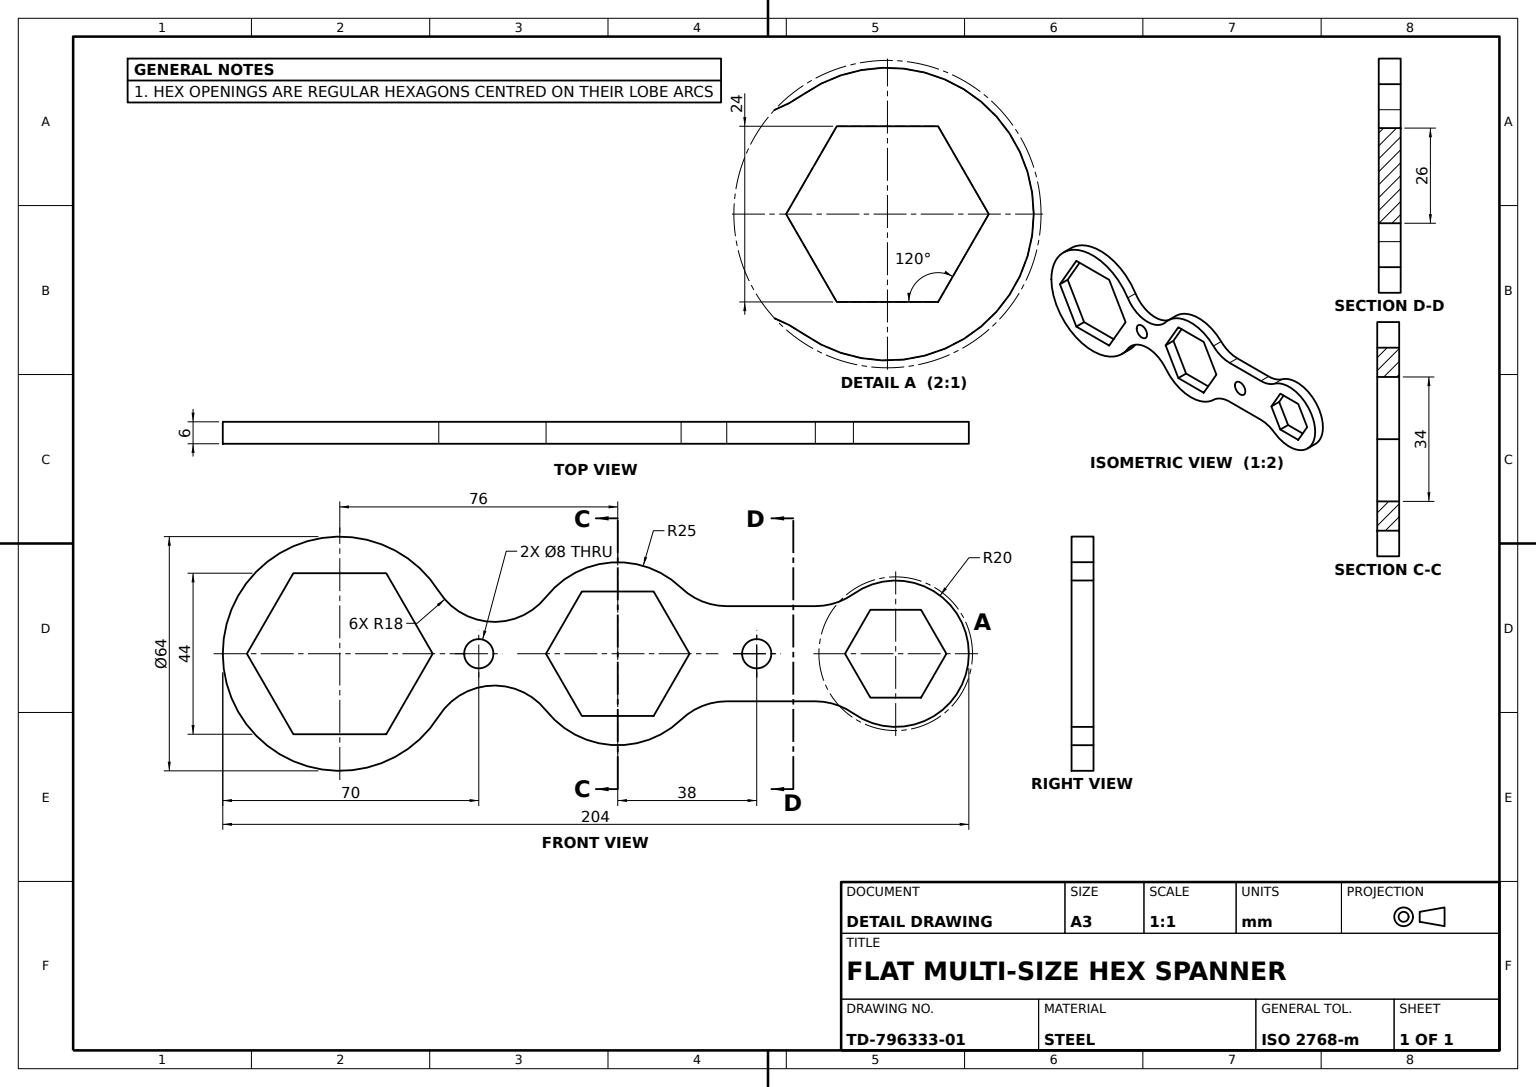
SolidWorks part; units mm, degrees
material "Plain Carbon Steel"
ref_plane "Front Plane" through (0, 0, 0) normal (0, 0, 1) x (1, 0, 0)
ref_plane "Top Plane" through (0, 0, 0) normal (0, 1, 0) x (1, 0, 0)
ref_plane "Right Plane" through (0, 0, 0) normal (1, 0, 0) x (0, 0, -1)
sketch "Spanner Outline Sketch" plane through (0, 0, 0) normal (0, 0, 1) x (1, 0, 0)
  line L0 (0, 0) -> (76, 0) construction
  line L1 (76, 0) -> (152, 0) construction
  line L2 (105.7993, -13) -> (130.0227, -13)
  line L3 (105.7993, 13) -> (130.0227, 13)
  line L5 (76, 13) -> (152, 13) construction
  line L6 (76, -13) -> (152, -13) construction
  arc A0 (27.0611, 17.0792) -> (27.0611, -17.0792) centre (0, 0) ccw
  arc A1 (56.397, -15.5153) -> (93.3252, -18.0233) centre (76, 0) ccw
  arc A2 (140.433, -16.3158) -> (140.433, 16.3158) centre (152, 0) ccw
  arc A3 (27.0611, 17.0792) -> (56.397, 15.5153) centre (42.2829, 26.6863) ccw
  arc A4 (56.397, -15.5153) -> (27.0611, -17.0792) centre (42.2829, -26.6863) ccw
  arc A5 (93.3252, 18.0233) -> (56.397, 15.5153) centre (76, 0) ccw
  arc A6 (93.3252, 18.0233) -> (105.7993, 13) centre (105.7993, 31) ccw
  arc A7 (130.0227, 13) -> (140.433, 16.3158) centre (130.0227, 31) ccw
  arc A8 (105.7993, -13) -> (93.3252, -18.0233) centre (105.7993, -31) ccw
  arc A9 (140.433, -16.3158) -> (130.0227, -13) centre (130.0227, -31) ccw
  dimension "D1" = 76
  dimension "D3" = 64
  dimension "D4" = 50
  dimension "D5" = 40
  dimension "D6" = 36
  dimension "D7" = 36
  dimension "D10" = 36
  dimension "D11" = 36
  dimension "D12" = 18
  dimension "D13" = 36
  dimension "D2" = 76
  dimension "D8" = 13
  dimension "D9" = 13
extrude "Spanner Plate 6mm" add sketch "Spanner Outline Sketch" along normal blind 6
sketch "Hex Openings Sketch" plane through (0, 0, 6) normal (0, 0, 1) x (1, 0, 0)
  line L0 (0, 0) -> (76, 0) construction
  line L1 (25.4034, 0) -> (12.7017, 22)
  line L2 (12.7017, 22) -> (-12.7017, 22)
  line L3 (-12.7017, 22) -> (-25.4034, 0)
  line L4 (-25.4034, 0) -> (-12.7017, -22)
  line L5 (-12.7017, -22) -> (12.7017, -22)
  line L6 (12.7017, -22) -> (25.4034, 0)
  line L7 (76, 0) -> (152, 0) construction
  line L8 (95.6299, 0) -> (85.815, 17)
  line L9 (85.815, 17) -> (66.185, 17)
  line L10 (66.185, 17) -> (56.3701, 0)
  line L11 (56.3701, 0) -> (66.185, -17)
  line L12 (66.185, -17) -> (85.815, -17)
  line L13 (85.815, -17) -> (95.6299, 0)
  line L15 (165.8564, 0) -> (158.9282, 12)
  line L16 (158.9282, 12) -> (145.0718, 12)
  line L17 (145.0718, 12) -> (138.1436, 0)
  line L18 (138.1436, 0) -> (145.0718, -12)
  line L19 (145.0718, -12) -> (158.9282, -12)
  line L20 (158.9282, -12) -> (165.8564, 0)
  circle A0 centre (0, 0) radius 22 construction
  circle A1 centre (76, 0) radius 17 construction
  circle A2 centre (152, 0) radius 12 construction
  dimension "D1" = 44
  dimension "D2" = 34
  dimension "D3" = 24
  dimension "D4" = 29.309
extrude "Hex Openings 44-34-24 AF" cut sketch "Hex Openings Sketch" against normal through all
sketch "Web Holes Sketch" plane through (0, 0, 6) normal (0, 0, 1) x (1, 0, 0)
  line L0 (56.3701, 0) -> (95.6299, 0) construction
  circle A0 centre (38, 0) radius 4
  circle A1 centre (114, 0) radius 4
  point P9 (76, 0)
  dimension "D1" = 8
  dimension "D2" = 8
  dimension "D3" = 38
  dimension "D4" = 38
extrude "Web Holes 2xØ8" cut sketch "Web Holes Sketch" against normal through all
